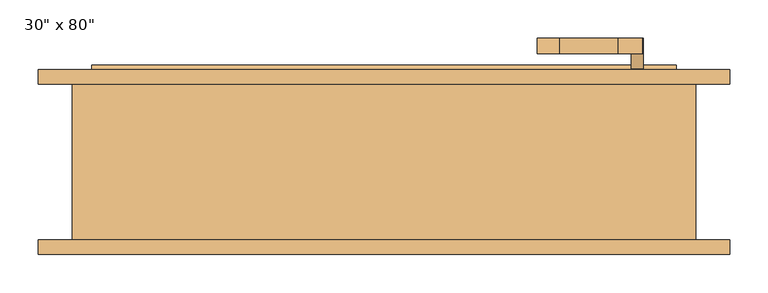
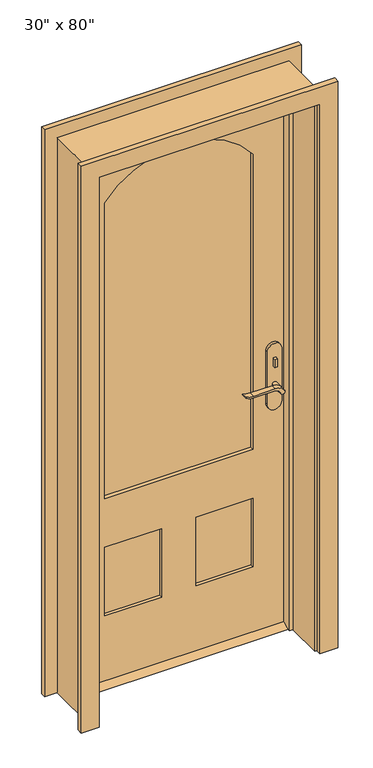
"""IFC4 building model written with IfcOpenShell, lengths in millimetres: door geometry."""

from ifc_helpers import new_model, si_unit, point, frame, frame_2d, origin, place, context, project, spatial, polyline, circle_curve, trimmed, segment, composite_curve, outline, extrude, faceted_brep, source, transform, mapped, element, save


def door_ad59dcae(model_context):
    return source(origin(), model_context, "Body", "SolidModel", [
        extrude(outline(polyline([(63.5, 12.7), (98.425, 12.7), (123.825, 0.0), (38.1, 0.0), (63.5, 12.7)])), frame((-381.0, 0.0, 0.0), z_axis=(1.0, 0.0, 0.0), x_axis=(0.0, 1.0, 0.0)), (0.0, 0.0, 1.0), 762.0),
        extrude(outline(polyline([(335.2, 43.5), (325.2, 43.5), (325.2, 53.5), (335.2, 53.5), (335.2, 43.5)])), frame((0.0, 0.0, 981.9), z_axis=(0.0, 0.0, 1.0), x_axis=(1.0, 0.0, 0.0)), (0.0, 0.0, 1.0), 30.0),
        extrude(outline(composite_curve([segment(trimmed(circle_curve(frame_2d((996.9, 330.2)), 8.0), [point((996.9, 322.2))], [point((996.9, 338.2))], False, "CARTESIAN"), True, "CONTINUOUS"), segment(trimmed(circle_curve(frame_2d((996.9, 330.2)), 8.0), [point((996.9, 338.2))], [point((996.9, 322.2))], False, "CARTESIAN"), True, "CONTINUOUS")], self_intersect=False)), frame((0.0, 108.425, 0.0), z_axis=(0.0, 1.0, 0.0), x_axis=(0.0, 0.0, 1.0)), (0.0, 0.0, 1.0), 10.0),
        extrude(outline(composite_curve([segment(trimmed(circle_curve(frame_2d((897.1555521, 306.5324871)), 37.2832219), [point((919.0523287, 336.7081363))], [point((934.4, 304.8325667))], False, "CARTESIAN"), True, "CONTINUOUS"), segment(polyline([(934.4, 304.8325667), (934.4, 228.5564091)]), True, "CONTINUOUS"), segment(trimmed(circle_curve(frame_2d((1017.6850638, 228.6227909)), 83.2850902), [point((934.4, 228.5564091))], [point((939.4, 200.2))], True, "CARTESIAN"), True, "CONTINUOUS"), segment(polyline([(939.4, 200.2), (936.6135558, 200.2)]), True, "CONTINUOUS"), segment(trimmed(circle_curve(frame_2d((986.6709207, 232.1396612)), 59.3791355), [point((936.6135558, 200.2))], [point((927.4, 228.5564091))], False, "CARTESIAN"), True, "CONTINUOUS"), segment(polyline([(927.4, 228.5564091), (927.4, 304.8138099)]), True, "CONTINUOUS"), segment(trimmed(circle_curve(frame_2d((909.2738613, 304.8138099)), 18.1261387), [point((927.4, 304.8138099))], [point((914.4, 322.2))], True, "CARTESIAN"), True, "CONTINUOUS"), segment(trimmed(circle_curve(frame_2d((914.4, 330.2)), 8.0), [point((914.4, 322.2))], [point((919.0523287, 336.7081363))], False, "CARTESIAN"), True, "CONTINUOUS")], self_intersect=False)), frame((0.0, 3.5, 0.0), z_axis=(0.0, 1.0, 0.0), x_axis=(0.0, 0.0, 1.0)), (0.0, 0.0, 1.0), 20.0),
        extrude(outline(composite_curve([segment(trimmed(circle_curve(frame_2d((914.4, 330.2)), 8.0), [point((914.3999903, 322.2))], [point((919.0523287, 336.7081363))], False, "CARTESIAN"), True, "CONTINUOUS"), segment(trimmed(circle_curve(frame_2d((897.1555521, 306.5324871)), 37.2832219), [point((919.0523287, 336.7081363))], [point((934.4, 304.8325667))], False, "CARTESIAN"), True, "CONTINUOUS"), segment(polyline([(934.4, 304.8325667), (934.4, 228.5564091)]), True, "CONTINUOUS"), segment(trimmed(circle_curve(frame_2d((1017.6850638, 228.6227909)), 83.2850902), [point((934.4, 228.5564091))], [point((939.4, 200.2))], True, "CARTESIAN"), True, "CONTINUOUS"), segment(polyline([(939.4, 200.2), (936.6135558, 200.2)]), True, "CONTINUOUS"), segment(trimmed(circle_curve(frame_2d((986.6709207, 232.1396612)), 59.3791355), [point((936.6135558, 200.2))], [point((927.4, 228.5564091))], False, "CARTESIAN"), True, "CONTINUOUS"), segment(polyline([(927.4, 228.5564091), (927.4, 304.8138122)]), True, "CONTINUOUS"), segment(trimmed(circle_curve(frame_2d((909.2738682, 304.8138122)), 18.1261318), [point((927.4, 304.8138122))], [point((914.3999903, 322.2))], True, "CARTESIAN"), True, "CONTINUOUS")], self_intersect=False)), frame((0.0, 138.425, 0.0), z_axis=(0.0, 1.0, 0.0), x_axis=(0.0, 0.0, 1.0)), (0.0, 0.0, 1.0), 20.0),
        extrude(outline(composite_curve([segment(trimmed(circle_curve(frame_2d((914.4, 330.2)), 8.0), [point((914.4, 322.2))], [point((914.4, 338.2))], False, "CARTESIAN"), True, "CONTINUOUS"), segment(trimmed(circle_curve(frame_2d((914.4, 330.2)), 8.0), [point((914.4, 338.2))], [point((914.4, 322.2))], False, "CARTESIAN"), True, "CONTINUOUS")], self_intersect=False)), frame((0.0, 23.5, 0.0), z_axis=(0.0, 1.0, 0.0), x_axis=(0.0, 0.0, 1.0)), (0.0, 0.0, 1.0), 30.0),
        extrude(outline(composite_curve([segment(trimmed(circle_curve(frame_2d((914.4, 330.2)), 8.0), [point((914.4, 322.2))], [point((914.4, 338.2))], False, "CARTESIAN"), True, "CONTINUOUS"), segment(trimmed(circle_curve(frame_2d((914.4, 330.2)), 8.0), [point((914.4, 338.2))], [point((914.4, 322.2))], False, "CARTESIAN"), True, "CONTINUOUS")], self_intersect=False)), frame((0.0, 108.425, 0.0), z_axis=(0.0, 1.0, 0.0), x_axis=(0.0, 0.0, 1.0)), (0.0, 0.0, 1.0), 30.0),
        extrude(outline(composite_curve([segment(polyline([(844.4, 355.2), (1039.4, 355.2)]), True, "CONTINUOUS"), segment(trimmed(circle_curve(frame_2d((1039.4, 330.2)), 25.0), [point((1039.4, 355.2))], [point((1039.4, 305.2))], False, "CARTESIAN"), True, "CONTINUOUS"), segment(polyline([(1039.4, 305.2), (844.4, 305.2)]), True, "CONTINUOUS"), segment(trimmed(circle_curve(frame_2d((844.4, 330.2)), 25.0), [point((844.4, 305.2))], [point((844.4, 355.2))], False, "CARTESIAN"), True, "CONTINUOUS")], self_intersect=False)), frame((0.0, 53.5, 0.0), z_axis=(0.0, 1.0, 0.0), x_axis=(0.0, 0.0, 1.0)), (0.0, 0.0, 1.0), 10.0),
        extrude(outline(composite_curve([segment(polyline([(844.4, 355.2), (1039.4, 355.2)]), True, "CONTINUOUS"), segment(trimmed(circle_curve(frame_2d((1039.4, 330.2)), 25.0), [point((1039.4, 355.2))], [point((1039.4, 305.2))], False, "CARTESIAN"), True, "CONTINUOUS"), segment(polyline([(1039.4, 305.2), (844.4, 305.2)]), True, "CONTINUOUS"), segment(trimmed(circle_curve(frame_2d((844.4, 330.2)), 25.0), [point((844.4, 305.2))], [point((844.4, 355.2))], False, "CARTESIAN"), True, "CONTINUOUS")], self_intersect=False)), frame((0.0, 98.425, 0.0), z_axis=(0.0, 1.0, 0.0), x_axis=(0.0, 0.0, 1.0)), (0.0, 0.0, 1.0), 10.0),
        extrude(outline(polyline([(2032.0, -381.0), (12.7, -381.0), (12.7, 381.0), (2032.0, 381.0), (2032.0, -381.0)]), holes=[composite_curve([segment(polyline([(688.975, -260.35), (1784.35, -260.35)]), True, "CONTINUOUS"), segment(trimmed(circle_curve(frame_2d((1580.99125, 0.0)), 330.35875), [point((1784.35, -260.35))], [point((1784.35, 260.35))], True, "CARTESIAN"), True, "CONTINUOUS"), segment(polyline([(1784.35, 260.35), (688.975, 260.35), (688.975, -260.35)]), True, "CONTINUOUS")], self_intersect=False), polyline([(508.0, -60.325), (254.0, -60.325), (254.0, -260.35), (508.0, -260.35), (508.0, -60.325)]), polyline([(508.0, 260.35), (254.0, 260.35), (254.0, 60.325), (508.0, 60.325), (508.0, 260.35)])]), frame((0.0, 63.5, 0.0), z_axis=(0.0, 1.0, 0.0), x_axis=(0.0, 0.0, 1.0)), (0.0, 0.0, 1.0), 34.925),
        faceted_brep([(406.4, 98.425, 0.0), (406.4, -104.775, 0.0), (381.0, -104.775, 0.0), (381.0, 28.575, 0.0), (368.3, 28.575, 0.0), (368.3, 63.5, 0.0), (381.0, 63.5, 0.0), (381.0, 98.425, 0.0), (406.4, 98.425, 2057.4), (406.4, -104.775, 2057.4), (-406.4, -104.775, 2057.4), (-406.4, -104.775, 0.0), (-381.0, -104.775, 0.0), (-381.0, -104.775, 2032.0), (381.0, -104.775, 2032.0), (381.0, 28.575, 2032.0), (-381.0, 28.575, 2032.0), (-381.0, 28.575, 0.0), (-368.3, 28.575, 0.0), (-368.3, 28.575, 2019.3), (368.3, 28.575, 2019.3), (368.3, 63.5, 2019.3), (-368.3, 63.5, 2019.3), (-368.3, 63.5, 0.0), (-381.0, 63.5, 0.0), (-381.0, 63.5, 2032.0), (381.0, 63.5, 2032.0), (381.0, 98.425, 2032.0), (-381.0, 98.425, 2032.0), (-381.0, 98.425, 0.0), (-406.4, 98.425, 0.0), (-406.4, 98.425, 2057.4)], [[[0, 1, 2, 3, 4, 5, 6, 7]], [[1, 0, 8, 9]], [[2, 1, 9, 10, 11, 12, 13, 14]], [[3, 2, 14, 15]], [[4, 3, 15, 16, 17, 18, 19, 20]], [[5, 4, 20, 21]], [[6, 5, 21, 22, 23, 24, 25, 26]], [[7, 6, 26, 27]], [[0, 7, 27, 28, 29, 30, 31, 8]], [[9, 8, 31, 10]], [[15, 14, 13, 16]], [[21, 20, 19, 22]], [[27, 26, 25, 28]], [[30, 29, 24, 23, 18, 17, 12, 11]], [[10, 31, 30, 11]], [[16, 13, 12, 17]], [[22, 19, 18, 23]], [[28, 25, 24, 29]]]),
        extrude(outline(polyline([(-60.325, 75.1416667), (-260.35, 75.1416667), (-260.35, 86.7833333), (-60.325, 86.7833333), (-60.325, 75.1416667)])), frame((0.0, 0.0, 254.0), z_axis=(0.0, 0.0, 1.0), x_axis=(1.0, 0.0, 0.0)), (0.0, 0.0, 1.0), 254.0),
        extrude(outline(polyline([(260.35, 75.1416667), (60.325, 75.1416667), (60.325, 86.7833333), (260.35, 86.7833333), (260.35, 75.1416667)])), frame((0.0, 0.0, 254.0), z_axis=(0.0, 0.0, 1.0), x_axis=(1.0, 0.0, 0.0)), (0.0, 0.0, 1.0), 254.0),
        extrude(outline(composite_curve([segment(polyline([(688.975, -260.35), (688.975, 260.35), (1784.35, 260.35)]), True, "CONTINUOUS"), segment(trimmed(circle_curve(frame_2d((1580.99125, 0.0)), 330.35875), [point((1784.35, 260.35))], [point((1784.35, -260.35))], False, "CARTESIAN"), True, "CONTINUOUS"), segment(polyline([(1784.35, -260.35), (688.975, -260.35)]), True, "CONTINUOUS")], self_intersect=False)), frame((0.0, 77.47, 0.0), z_axis=(0.0, 1.0, 0.0), x_axis=(0.0, 0.0, 1.0)), (0.0, 0.0, 1.0), 6.985),
        extrude(outline(polyline([(0.0, -450.85), (0.0, -387.35), (2038.35, -387.35), (2038.35, 387.35), (0.0, 387.35), (0.0, 450.85), (2101.85, 450.85), (2101.85, -450.85), (0.0, -450.85)])), frame((0.0, -123.825, 0.0), z_axis=(0.0, 1.0, 0.0), x_axis=(0.0, 0.0, 1.0)), (0.0, 0.0, 1.0), 19.05),
        extrude(outline(polyline([(0.0, -450.85), (0.0, -387.35), (2038.35, -387.35), (2038.35, 387.35), (0.0, 387.35), (0.0, 450.85), (2101.85, 450.85), (2101.85, -450.85), (0.0, -450.85)])), frame((0.0, 98.425, 0.0), z_axis=(0.0, 1.0, 0.0), x_axis=(0.0, 0.0, 1.0)), (0.0, 0.0, 1.0), 19.05),
    ])


if __name__ == "__main__":
    model = new_model("IFC4")
    model_context = context("Model", 3, world=origin())
    ifc_project = project(units=[si_unit("LENGTHUNIT", "METRE", prefix="MILLI")], contexts=[model_context])
    site = spatial("IfcSite", under=ifc_project)
    building = spatial("IfcBuilding", under=site)
    placement = place(None, origin())
    door_shape = door_ad59dcae(model_context)
    element("IfcDoor", 1, ObjectType="30\" x 80\"", at=placement, inside=building, context=model_context, shape_type="MappedRepresentation", body=[
        mapped(door_shape, transform((0.0, 0.0, 0.0), x_axis=(1.0, 0.0, 0.0), y_axis=(0.0, 1.0, 0.0), z_axis=(0.0, 0.0, 1.0))),
    ])
    save(model, "model.ifc")

# Revit data of these elements
# Type "30\" x 80\""
#   Type Mark = "11"
#   Assembly Code = "B2030100"
#   Analytic Construction = "French door, wood frame with single glass"
#   Threshold Offset [instance default] = 0' - 0 1/2"
#   Thickness = 0' - 1 3/8"
#   Thermal Resistance (R) = 1.0696 (h·ft²·°F)/BTU
#   Swing Angle [instance default] = 90.00°
#   Stiles = 0' - 4 3/4"
#   Rough Width = 2' - 8"
#   Rough Height = 6' - 9"
#   Radius = 1' - 1.00625"
#   Lock Rail = 0' - 7 1/8"
#   Height = 6' - 8"
#   Width = 2' - 6"
#   Heat Transfer Coefficient (U) = 0.9350 BTU/(h·ft²·°F)
#   Door Offset [instance default] = 0' - 0"
#   Bottom Rail = 0' - 9 1/2"
#   Threshold [instance default] = yes
#   Function = 1
#   Exterior Trim [instance default] = yes
#   Trim Material = Cherry
#   Threshold Material = Cherry
#   Panel Material = Cherry
#   Glazing = Glass
#   Frame Material = Cherry
#   Door Handle Material = Aluminum
#   Visual Light Transmittance = 0
#   Solar Heat Gain Coefficient = 0
#   Wall Closure = (empty or 0)
#   Construction Type = (empty or 0)
# Element 1 (IfcDoor, "30\" x 80\"")
#   Materials on its faces: "Cherry", "Aluminum", "Glass"
# Materials
#   "Cherry": class "Wood", colour RGB 226 177 128, transparency 0, Description = "Prunus Serotina", Cost = 0
#   "Glass": class "Glass", colour RGB 0 128 192, transparency 0.75, Description = "Soda Lime Glass", Cost = 0
#   "Aluminum": class "Metal", colour RGB 247 247 247, transparency 0, Description = "Aluminum 6061", Cost = 0
